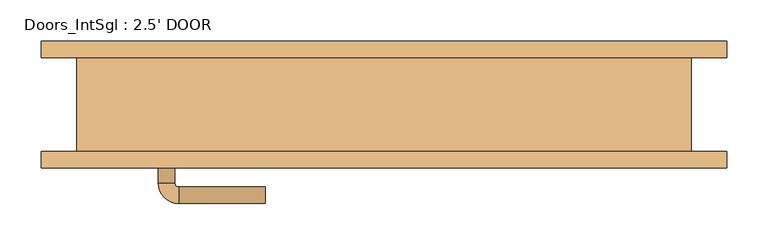
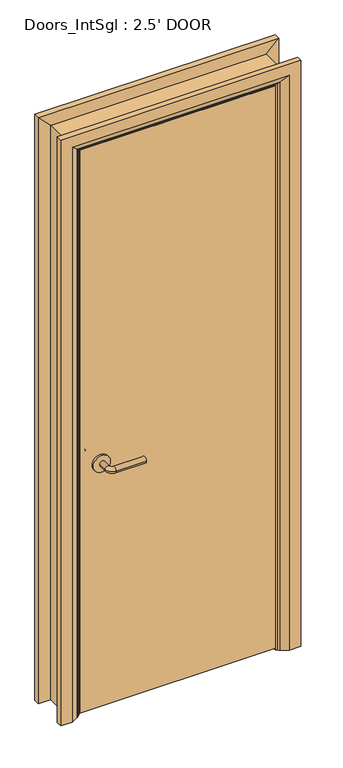
"""IFC4 building model written with IfcOpenShell, lengths in millimetres: door geometry, Doors_IntSgl : 2.5' DOOR."""

from ifc_helpers import new_model, si_unit, point, frame, frame_2d, origin, place, context, project, spatial, polyline, circle_curve, ellipse_curve, trimmed, segment, composite_curve, outline, extrude, faceted_brep, source, transform, mapped, element, save
from ifc_brep_helpers import plane_surface, cylinder_surface, revolved_surface, advanced_brep


def doors_intsgl_2_5_door_1f5f3f16(model_context):
    return source(origin(), model_context, "Body", "SolidModel", [
        advanced_brep(
        [(-274.0, -11.15, 900.0), (-254.0, -11.15, 900.0), (-274.0, 18.85, 900.0), (-254.0, 18.85, 900.0), (-249.0, 23.85, 900.0), (-249.0, 43.85, 900.0), (-144.0, 43.85, 900.0), (-144.0, 23.85, 900.0)],
        [
            (0, 1, circle_curve(frame((-264.0, -11.15, 900.0), z_axis=(0.0, -1.0, 0.0), x_axis=(1.0, 0.0, 0.0)), 10.0)),
            (1, 0, circle_curve(frame((-264.0, -11.15, 900.0), z_axis=(0.0, -1.0, 0.0), x_axis=(1.0, 0.0, 0.0)), 10.0)),
            (0, 2),
            (2, 3, circle_curve(frame((-264.0, 18.85, 900.0), z_axis=(0.0, -1.0, 0.0), x_axis=(1.0, 0.0, 0.0)), 10.0)),
            (3, 1),
            (3, 2, circle_curve(frame((-264.0, 18.85, 900.0), z_axis=(0.0, -1.0, 0.0), x_axis=(1.0, 0.0, 0.0)), 10.0)),
            (4, 3, circle_curve(frame((-249.0, 18.85, 900.0), z_axis=(0.0, 0.0, 1.0), x_axis=(-1.0, 0.0, 0.0)), 5.0)),
            (2, 5, circle_curve(frame((-249.0, 18.85, 900.0), z_axis=(0.0, 0.0, -1.0), x_axis=(-1.0, 0.0, 0.0)), 25.0)),
            (5, 4, circle_curve(frame((-249.0, 33.85, 900.0), z_axis=(-1.0, 0.0, 0.0), x_axis=(0.0, -1.0, 0.0)), 10.0)),
            (4, 5, circle_curve(frame((-249.0, 33.85, 900.0), z_axis=(-1.0, 0.0, 0.0), x_axis=(0.0, -1.0, 0.0)), 10.0)),
            (6, 7, circle_curve(frame((-144.0, 33.85, 900.0), z_axis=(1.0, 0.0, 0.0), x_axis=(0.0, -1.0, 0.0)), 10.0)),
            (7, 6, circle_curve(frame((-144.0, 33.85, 900.0), z_axis=(1.0, 0.0, 0.0), x_axis=(0.0, -1.0, 0.0)), 10.0)),
            (5, 6),
            (7, 4),
        ],
        [
            plane_surface(frame((-264.0, -11.15, 900.0), z_axis=(0.0, -1.0, 0.0), x_axis=(0.0, 0.0, 1.0))),
            cylinder_surface(frame((-264.0, -11.15, 900.0), z_axis=(0.0, -1.0, 0.0), x_axis=(1.0, 0.0, 0.0)), 10.0),
            revolved_surface(trimmed(ellipse_curve(frame((-264.0, 18.85, 900.0), z_axis=(0.0, -1.0, 0.0), x_axis=(1.0, 0.0, 0.0)), 10.0, 10.0), [point((-274.0, 18.85, 900.0))], [point((-254.0, 18.85, 900.0))], True, "CARTESIAN"), (-249.0, 18.85, 900.0), (0.0, 0.0, -1.0)),
            revolved_surface(trimmed(ellipse_curve(frame((-264.0, 18.85, 900.0), z_axis=(0.0, -1.0, 0.0), x_axis=(1.0, 0.0, 0.0)), 10.0, 10.0), [point((-254.0, 18.85, 900.0))], [point((-274.0, 18.85, 900.0))], True, "CARTESIAN"), (-249.0, 18.85, 900.0), (0.0, 0.0, -1.0)),
            plane_surface(frame((-144.0, 33.85, 900.0), z_axis=(1.0, 0.0, 0.0), x_axis=(0.0, 0.0, 1.0))),
            cylinder_surface(frame((-249.0, 33.85, 900.0), z_axis=(-1.0, 0.0, 0.0), x_axis=(0.0, -1.0, 0.0)), 10.0),
        ],
        [
            (0, [[1, 2]]),
            (1, [[-1, 3, 4, 5]]),
            (1, [[-2, -5, 6, -3]]),
            (2, [[7, -4, 8, 9]]),
            (3, [[-8, -6, -7, 10]]),
            (4, [[11, 12]]),
            (5, [[-9, 13, -12, 14]]),
            (5, [[-10, -14, -11, -13]]),
        ],
    ),
        extrude(outline(composite_curve([segment(trimmed(circle_curve(frame_2d((900.0, -266.5)), 30.0), [point((900.0, -296.5))], [point((900.0, -236.5))], False, "CARTESIAN"), True, "CONTINUOUS"), segment(trimmed(circle_curve(frame_2d((900.0, -266.5)), 30.0), [point((900.0, -236.5))], [point((900.0, -296.5))], False, "CARTESIAN"), True, "CONTINUOUS")], self_intersect=False)), frame((0.0, -19.15, 0.0), z_axis=(0.0, 1.0, 0.0), x_axis=(0.0, 0.0, 1.0)), (0.0, 0.0, 1.0), 8.0),
        advanced_brep(
        [(-274.0, -65.15, 900.0), (-254.0, -65.15, 900.0), (-254.0, -95.15, 900.0), (-274.0, -95.15, 900.0), (-249.0, -100.15, 900.0), (-249.0, -120.15, 900.0), (-144.0, -120.15, 900.0), (-144.0, -100.15, 900.0)],
        [
            (0, 1, circle_curve(frame((-264.0, -65.15, 900.0), z_axis=(0.0, 1.0, 0.0), x_axis=(1.0, 0.0, 0.0)), 10.0)),
            (1, 0, circle_curve(frame((-264.0, -65.15, 900.0), z_axis=(0.0, 1.0, 0.0), x_axis=(1.0, 0.0, 0.0)), 10.0)),
            (1, 2),
            (2, 3, circle_curve(frame((-264.0, -95.15, 900.0), z_axis=(0.0, 1.0, 0.0), x_axis=(1.0, 0.0, 0.0)), 10.0)),
            (3, 0),
            (3, 2, circle_curve(frame((-264.0, -95.15, 900.0), z_axis=(0.0, 1.0, 0.0), x_axis=(1.0, 0.0, 0.0)), 10.0)),
            (4, 5, circle_curve(frame((-249.0, -110.15, 900.0), z_axis=(-1.0, 0.0, 0.0), x_axis=(0.0, 1.0, 0.0)), 10.0)),
            (5, 3, circle_curve(frame((-249.0, -95.15, 900.0), z_axis=(0.0, 0.0, -1.0), x_axis=(-1.0, 0.0, 0.0)), 25.0)),
            (2, 4, circle_curve(frame((-249.0, -95.15, 900.0), z_axis=(0.0, 0.0, 1.0), x_axis=(-1.0, 0.0, 0.0)), 5.0)),
            (5, 4, circle_curve(frame((-249.0, -110.15, 900.0), z_axis=(-1.0, 0.0, 0.0), x_axis=(0.0, 1.0, 0.0)), 10.0)),
            (6, 7, circle_curve(frame((-144.0, -110.15, 900.0), z_axis=(1.0, 0.0, 0.0), x_axis=(0.0, 1.0, 0.0)), 10.0)),
            (7, 6, circle_curve(frame((-144.0, -110.15, 900.0), z_axis=(1.0, 0.0, 0.0), x_axis=(0.0, 1.0, 0.0)), 10.0)),
            (4, 7),
            (6, 5),
        ],
        [
            plane_surface(frame((-264.0, -65.15, 900.0), z_axis=(0.0, 1.0, 0.0), x_axis=(0.0, 0.0, 1.0))),
            cylinder_surface(frame((-264.0, -65.15, 900.0), z_axis=(0.0, 1.0, 0.0), x_axis=(1.0, 0.0, 0.0)), 10.0),
            revolved_surface(trimmed(ellipse_curve(frame((-264.0, -95.15, 900.0), z_axis=(0.0, -1.0, 0.0), x_axis=(1.0, 0.0, 0.0)), 10.0, 10.0), [point((-274.0, -95.15, 900.0))], [point((-254.0, -95.15, 900.0))], True, "CARTESIAN"), (-249.0, -95.15, 900.0), (0.0, 0.0, -1.0)),
            revolved_surface(trimmed(ellipse_curve(frame((-264.0, -95.15, 900.0), z_axis=(0.0, -1.0, 0.0), x_axis=(1.0, 0.0, 0.0)), 10.0, 10.0), [point((-254.0, -95.15, 900.0))], [point((-274.0, -95.15, 900.0))], True, "CARTESIAN"), (-249.0, -95.15, 900.0), (0.0, 0.0, -1.0)),
            plane_surface(frame((-144.0, -110.15, 900.0), z_axis=(1.0, 0.0, 0.0), x_axis=(0.0, 0.0, 1.0))),
            cylinder_surface(frame((-249.0, -110.15, 900.0), z_axis=(-1.0, 0.0, 0.0), x_axis=(0.0, 1.0, 0.0)), 10.0),
        ],
        [
            (0, [[1, 2]]),
            (1, [[3, 4, 5, -2]]),
            (1, [[-5, 6, -3, -1]]),
            (2, [[7, 8, -4, 9]]),
            (3, [[10, -9, -6, -8]]),
            (4, [[11, 12]]),
            (5, [[13, -11, 14, -7]]),
            (5, [[-14, -12, -13, -10]]),
        ],
    ),
        extrude(outline(composite_curve([segment(trimmed(circle_curve(frame_2d((900.0, -266.5)), 30.0), [point((900.0, -296.5))], [point((900.0, -236.5))], False, "CARTESIAN"), True, "CONTINUOUS"), segment(trimmed(circle_curve(frame_2d((900.0, -266.5)), 30.0), [point((900.0, -236.5))], [point((900.0, -296.5))], False, "CARTESIAN"), True, "CONTINUOUS")], self_intersect=False)), frame((0.0, -65.15, 0.0), z_axis=(0.0, 1.0, 0.0), x_axis=(0.0, 0.0, 1.0)), (0.0, 0.0, 1.0), 8.0),
        extrude(outline(polyline([(339.0, -19.15), (339.0, -57.15), (-339.0, -57.15), (-339.0, -19.15), (339.0, -19.15)])), frame((0.0, 0.0, 8.0), z_axis=(0.0, 0.0, 1.0), x_axis=(1.0, 0.0, 0.0)), (0.0, 0.0, 1.0), 2060.0),
        advanced_brep(
        [(416.0, -77.15, 0.0), (376.0, -77.15, 0.0), (350.0, -63.15, 0.0), (346.0, -57.15, 0.0), (416.0, -57.15, 0.0), (416.0, -57.15, 2145.0), (416.0, -77.15, 2145.0), (346.0, -57.15, 2075.0), (-346.0, -57.15, 2075.0), (-346.0, -57.15, 0.0), (-416.0, -57.15, 0.0), (-416.0, -57.15, 2145.0), (350.0, -63.15, 2079.0), (376.0, -77.15, 2105.0), (-416.0, -77.15, 2145.0), (-416.0, -77.15, 0.0), (-376.0, -77.15, 0.0), (-376.0, -77.15, 2105.0), (-350.0, -63.15, 0.0), (-350.0, -63.15, 2079.0)],
        [
            (0, 1),
            (1, 2),
            (2, 3, circle_curve(frame((354.0, -56.15, 0.0), z_axis=(0.0, 0.0, -1.0), x_axis=(1.0, 0.0, 0.0)), 8.0622577)),
            (3, 4),
            (4, 0),
            (4, 5),
            (5, 6),
            (6, 0),
            (3, 7),
            (7, 8),
            (8, 9),
            (9, 10),
            (10, 11),
            (11, 5),
            (2, 12),
            (12, 7, ellipse_curve(frame((354.0, -56.15, 2083.0), z_axis=(0.7071067811865475, 0.0, -0.7071067811865475), x_axis=(-0.7071067811865474, 0.0, -0.7071067811865476)), 11.4017543, 8.0622577)),
            (1, 13),
            (13, 12),
            (6, 14),
            (14, 15),
            (15, 16),
            (16, 17),
            (17, 13),
            (10, 15),
            (14, 11),
            (9, 18, circle_curve(frame((-354.0, -56.15, 0.0), z_axis=(0.0, 0.0, -1.0), x_axis=(-1.0, 0.0, 0.0)), 8.0622577)),
            (18, 16),
            (19, 18),
            (8, 19, ellipse_curve(frame((-354.0, -56.15, 2083.0), z_axis=(-0.7071067811865475, 0.0, -0.7071067811865475), x_axis=(-0.7071067811865474, 0.0, 0.7071067811865476)), 11.4017543, 8.0622577)),
            (19, 17),
            (12, 19),
        ],
        [
            plane_surface(frame((346.0, -57.15, 0.0), z_axis=(0.0, 0.0, -1.0), x_axis=(0.0, 1.0, 0.0))),
            plane_surface(frame((416.0, -77.15, 0.0), z_axis=(1.0, 0.0, 0.0), x_axis=(0.0, 0.0, 1.0))),
            plane_surface(frame((416.0, -57.15, 0.0), z_axis=(0.0, 1.0, 0.0), x_axis=(0.0, 0.0, 1.0))),
            cylinder_surface(frame((354.0, -56.15, 0.0), z_axis=(0.0, 0.0, -1.0), x_axis=(1.0, 0.0, 0.0)), 8.0622577),
            plane_surface(frame((350.0, -63.15, 0.0), z_axis=(-0.4740998230350126, -0.880471099922178, 0.0), x_axis=(0.0, 0.0, 1.0))),
            plane_surface(frame((376.0, -77.15, 0.0), z_axis=(0.0, -1.0, 0.0), x_axis=(0.0, 0.0, 1.0))),
            plane_surface(frame((-416.0, -77.15, 2145.0), z_axis=(-1.0, 0.0, 0.0), x_axis=(0.0, 0.0, -1.0))),
            plane_surface(frame((-346.0, -57.15, 0.0), z_axis=(0.0, 0.0, -1.0), x_axis=(0.0, 1.0, 0.0))),
            cylinder_surface(frame((-354.0, -56.15, 2075.0), z_axis=(0.0, 0.0, 1.0), x_axis=(-1.0, 0.0, 0.0)), 8.0622577),
            plane_surface(frame((-350.0, -63.15, 2079.0), z_axis=(0.47409982303501824, -0.8804710999221749, 0.0), x_axis=(0.0, 0.0, -1.0))),
            plane_surface(frame((416.0, -77.15, 2145.0), z_axis=(0.0, 0.0, 1.0), x_axis=(-1.0, 0.0, 0.0))),
            cylinder_surface(frame((346.0, -56.15, 2083.0), z_axis=(1.0, 0.0, 0.0), x_axis=(0.0, 0.0, 1.0)), 8.0622577),
            plane_surface(frame((350.0, -63.15, 2079.0), z_axis=(0.0, -0.8804710999221764, -0.4740998230350154), x_axis=(-1.0, 0.0, 0.0))),
        ],
        [
            (0, [[1, 2, 3, 4, 5]]),
            (1, [[6, 7, 8, -5]]),
            (2, [[9, 10, 11, 12, 13, 14, -6, -4]]),
            (3, [[15, 16, -9, -3]]),
            (4, [[17, 18, -15, -2]]),
            (5, [[-8, 19, 20, 21, 22, 23, -17, -1]]),
            (6, [[-13, 24, -20, 25]]),
            (7, [[-24, -12, 26, 27, -21]]),
            (8, [[28, -26, -11, 29]]),
            (9, [[-22, -27, -28, 30]]),
            (10, [[-14, -25, -19, -7]]),
            (11, [[31, -29, -10, -16]]),
            (12, [[-23, -30, -31, -18]]),
        ],
    ),
        extrude(outline(polyline([(0.0, -322.0), (2051.0, -322.0), (2051.0, 322.0), (0.0, 322.0), (0.0, 341.0), (2070.0, 341.0), (2070.0, -341.0), (0.0, -341.0), (0.0, -322.0)])), frame((0.0, -17.15, 0.0), z_axis=(0.0, 1.0, 0.0), x_axis=(0.0, 0.0, 1.0)), (0.0, 0.0, 1.0), 32.0),
        advanced_brep(
        [(-416.0, 77.15, 0.0), (-376.0, 77.15, 0.0), (-350.0, 63.15, 0.0), (-346.0, 57.15, 0.0), (-416.0, 57.15, 0.0), (-416.0, 57.15, 2145.0), (-416.0, 77.15, 2145.0), (-346.0, 57.15, 2075.0), (-350.0, 63.15, 2079.0), (-376.0, 77.15, 2105.0), (416.0, 77.15, 0.0), (416.0, 57.15, 0.0), (346.0, 57.15, 0.0), (350.0, 63.15, 0.0), (376.0, 77.15, 0.0), (416.0, 77.15, 2145.0), (376.0, 77.15, 2105.0), (350.0, 63.15, 2079.0), (346.0, 57.15, 2075.0), (416.0, 57.15, 2145.0)],
        [
            (0, 1),
            (1, 2),
            (2, 3, circle_curve(frame((-354.0, 56.15, 0.0), z_axis=(0.0, 0.0, -1.0), x_axis=(-1.0, 0.0, 0.0)), 8.0622577)),
            (3, 4),
            (4, 0),
            (4, 5),
            (5, 6),
            (6, 0),
            (3, 7),
            (7, 5),
            (2, 8),
            (8, 7, ellipse_curve(frame((-354.0, 56.15, 2083.0), z_axis=(-0.7071067811865475, 0.0, -0.7071067811865475), x_axis=(0.7071067811865474, 0.0, -0.7071067811865476)), 11.4017543, 8.0622577)),
            (1, 9),
            (9, 8),
            (6, 9),
            (10, 11),
            (11, 12),
            (12, 13, circle_curve(frame((354.0, 56.15, 0.0), z_axis=(0.0, 0.0, -1.0), x_axis=(1.0, 0.0, 0.0)), 8.0622577)),
            (13, 14),
            (14, 10),
            (15, 10),
            (14, 16),
            (16, 15),
            (13, 17),
            (17, 16),
            (12, 18),
            (18, 17, ellipse_curve(frame((354.0, 56.15, 2083.0), z_axis=(0.7071067811865475, 0.0, -0.7071067811865475), x_axis=(0.7071067811865474, 0.0, 0.7071067811865476)), 11.4017543, 8.0622577)),
            (11, 19),
            (19, 18),
            (15, 19),
            (5, 19),
            (15, 6),
            (7, 18),
            (8, 17),
            (9, 16),
        ],
        [
            plane_surface(frame((-346.0, 129.9510989, 0.0), z_axis=(0.0, 0.0, -1.0), x_axis=(1.0, 0.0, 0.0))),
            plane_surface(frame((-416.0, 77.15, 0.0), z_axis=(-1.0, 0.0, 0.0), x_axis=(0.0, 0.0, 1.0))),
            plane_surface(frame((-416.0, 57.15, 0.0), z_axis=(0.0, -1.0, 0.0), x_axis=(0.0, 0.0, 1.0))),
            cylinder_surface(frame((-354.0, 56.15, 0.0), z_axis=(0.0, 0.0, -1.0), x_axis=(-1.0, 0.0, 0.0)), 8.0622577),
            plane_surface(frame((-350.0, 63.15, 0.0), z_axis=(0.4740998230350183, 0.8804710999221749, 0.0), x_axis=(0.0, 0.0, 1.0))),
            plane_surface(frame((-376.0, 77.15, 0.0), z_axis=(0.0, 1.0, 0.0), x_axis=(0.0, 0.0, 1.0))),
            plane_surface(frame((346.0, 129.9510989, 0.0), z_axis=(0.0, 0.0, -1.0), x_axis=(-1.0, 0.0, 0.0))),
            plane_surface(frame((376.0, 77.15, 2105.0), z_axis=(0.0, 1.0, 0.0), x_axis=(0.0, 0.0, -1.0))),
            plane_surface(frame((350.0, 63.15, 2079.0), z_axis=(-0.4740998230350183, 0.8804710999221749, 0.0), x_axis=(0.0, 0.0, -1.0))),
            cylinder_surface(frame((354.0, 56.15, 2075.0), z_axis=(0.0, 0.0, 1.0), x_axis=(1.0, 0.0, 0.0)), 8.0622577),
            plane_surface(frame((416.0, 57.15, 2145.0), z_axis=(0.0, -1.0, 0.0), x_axis=(0.0, 0.0, -1.0))),
            plane_surface(frame((416.0, 77.15, 2145.0), z_axis=(1.0, 0.0, 0.0), x_axis=(0.0, 0.0, -1.0))),
            plane_surface(frame((-416.0, 77.15, 2145.0), z_axis=(0.0, 0.0, 1.0), x_axis=(1.0, 0.0, 0.0))),
            plane_surface(frame((-416.0, 57.15, 2145.0), z_axis=(0.0, -1.0, 0.0), x_axis=(1.0, 0.0, 0.0))),
            cylinder_surface(frame((-346.0, 56.15, 2083.0), z_axis=(-1.0, 0.0, 0.0), x_axis=(0.0, 0.0, 1.0)), 8.0622577),
            plane_surface(frame((-350.0, 63.15, 2079.0), z_axis=(0.0, 0.8804710999221749, -0.4740998230350183), x_axis=(1.0, 0.0, 0.0))),
            plane_surface(frame((-376.0, 77.15, 2105.0), z_axis=(0.0, 1.0, 0.0), x_axis=(1.0, 0.0, 0.0))),
        ],
        [
            (0, [[1, 2, 3, 4, 5]]),
            (1, [[6, 7, 8, -5]]),
            (2, [[9, 10, -6, -4]]),
            (3, [[11, 12, -9, -3]]),
            (4, [[13, 14, -11, -2]]),
            (5, [[-8, 15, -13, -1]]),
            (6, [[16, 17, 18, 19, 20]]),
            (7, [[21, -20, 22, 23]]),
            (8, [[-22, -19, 24, 25]]),
            (9, [[-24, -18, 26, 27]]),
            (10, [[-26, -17, 28, 29]]),
            (11, [[-28, -16, -21, 30]]),
            (12, [[31, -30, 32, -7]]),
            (13, [[33, -29, -31, -10]]),
            (14, [[34, -27, -33, -12]]),
            (15, [[35, -25, -34, -14]]),
            (16, [[-32, -23, -35, -15]]),
        ],
    ),
        faceted_brep([(-341.0, -57.15, 0.0), (-373.0, -57.15, 0.0), (-373.0, 57.15, 0.0), (-341.0, 57.15, 0.0), (-341.0, 57.15, 2070.0), (-341.0, -57.15, 2070.0), (-373.0, 57.15, 2102.0), (-373.0, -57.15, 2102.0), (341.0, -57.15, 0.0), (341.0, 57.15, 0.0), (373.0, 57.15, 0.0), (373.0, -57.15, 0.0), (341.0, -57.15, 2070.0), (373.0, -57.15, 2102.0), (373.0, 57.15, 2102.0), (341.0, 57.15, 2070.0)], [[[0, 1, 2, 3]], [[3, 4, 5, 0]], [[2, 6, 4, 3]], [[1, 7, 6, 2]], [[0, 5, 7, 1]], [[8, 9, 10, 11]], [[12, 8, 11, 13]], [[13, 11, 10, 14]], [[14, 10, 9, 15]], [[15, 9, 8, 12]], [[4, 15, 12, 5]], [[6, 14, 15, 4]], [[7, 13, 14, 6]], [[5, 12, 13, 7]]]),
    ])


if __name__ == "__main__":
    model = new_model("IFC4")
    model_context = context("Model", 3, world=origin())
    ifc_project = project(units=[si_unit("LENGTHUNIT", "METRE", prefix="MILLI")], contexts=[model_context])
    site = spatial("IfcSite", under=ifc_project)
    building = spatial("IfcBuilding", under=site)
    placement = place(None, origin())
    doors_intsgl_2_5_door_shape = doors_intsgl_2_5_door_1f5f3f16(model_context)
    element("IfcDoor", 1, ObjectType="Doors_IntSgl : 2.5' DOOR", at=placement, inside=building, context=model_context, shape_type="MappedRepresentation", body=[
        mapped(doors_intsgl_2_5_door_shape, transform((0.0, 0.0, 0.0), x_axis=(1.0, 0.0, 0.0), y_axis=(0.0, 1.0, 0.0), z_axis=(0.0, 0.0, 1.0))),
    ])
    save(model, "model.ifc")

# Revit data of these elements
# Type "Doors_IntSgl : 2.5' DOOR"
#   Type Mark = "47"
#   Type Comments = "Internal Single"
#   Operation = "SingleSwingRight"
#   Manufacturer = "Revit"
#   Keynote = "L20"
#   Description = "Internal Single Door"
#   Analytic Construction = "Metal"
#   UnderCut = 0.026247 ft
#   Tolerance = 0.006562 ft
#   Thickness = 0.124672 ft
#   Thermal Resistance (R) = 0.270117 (m²·K)/W
#   Structural Tolerance = 0.026247 ft
#   StopDepth = 0.104987 ft
#   Stop Thickness = 0.062336 ft
#   Rough Width = 2.5 ft
#   Rough Height = 6.922572 ft
#   Height to Top Lock Rail = 3.28084 ft
#   Heat Transfer Coefficient (U) = 3.7021 W/(m²·K)
#   Handle Z Distance = 2.952756 ft
#   Handle X Distance = 0.246063 ft
#   Frame Thickness = 0.104987 ft
#   Door Panel Width = 2.224409 ft
#   Door Panel Thickness = 0.124672 ft
#   Door Panel Offset = 0.0 ft
#   Height = 6.922572 ft
#   Width = 2.5 ft
#   Door Panel Height = 6.75853 ft
#   Architrave Setback = 0.016404 ft
#   Vis - Ironmongery = yes
#   Material Ironmongery = Door - Handle
#   Material Frame = Door - Frame/Mullion (1)
#   Material Door = Door - Panel
#   Material Architrave = Door - Architrave
#   Visual Light Transmittance = 0
#   Solar Heat Gain Coefficient = 0
#   Function = (empty or 0)
#   Wall Closure = (empty or 0)
# Element 1 (IfcDoor, "Doors_IntSgl : 2.5' DOOR")
#   Materials on its faces: "Door - Architrave", "Door - Handle", "Door - Frame/Mullion (1)", "Door - Panel"
# Materials
#   "Door - Handle": colour RGB 0 0 0, transparency 0, Keynote = "P21", Cost = 0
#   "Door - Frame/Mullion (1)": class "Wood", colour RGB 212 179 113, transparency 0, Keynote = "L20", Cost = 0
#   "Door - Panel": class "Wood", colour RGB 210 159 95, transparency 0, Keynote = "L20", Cost = 0
#   "Door - Architrave": class "Wood", colour RGB 154 90 5, transparency 0, Keynote = "P20", Cost = 0
